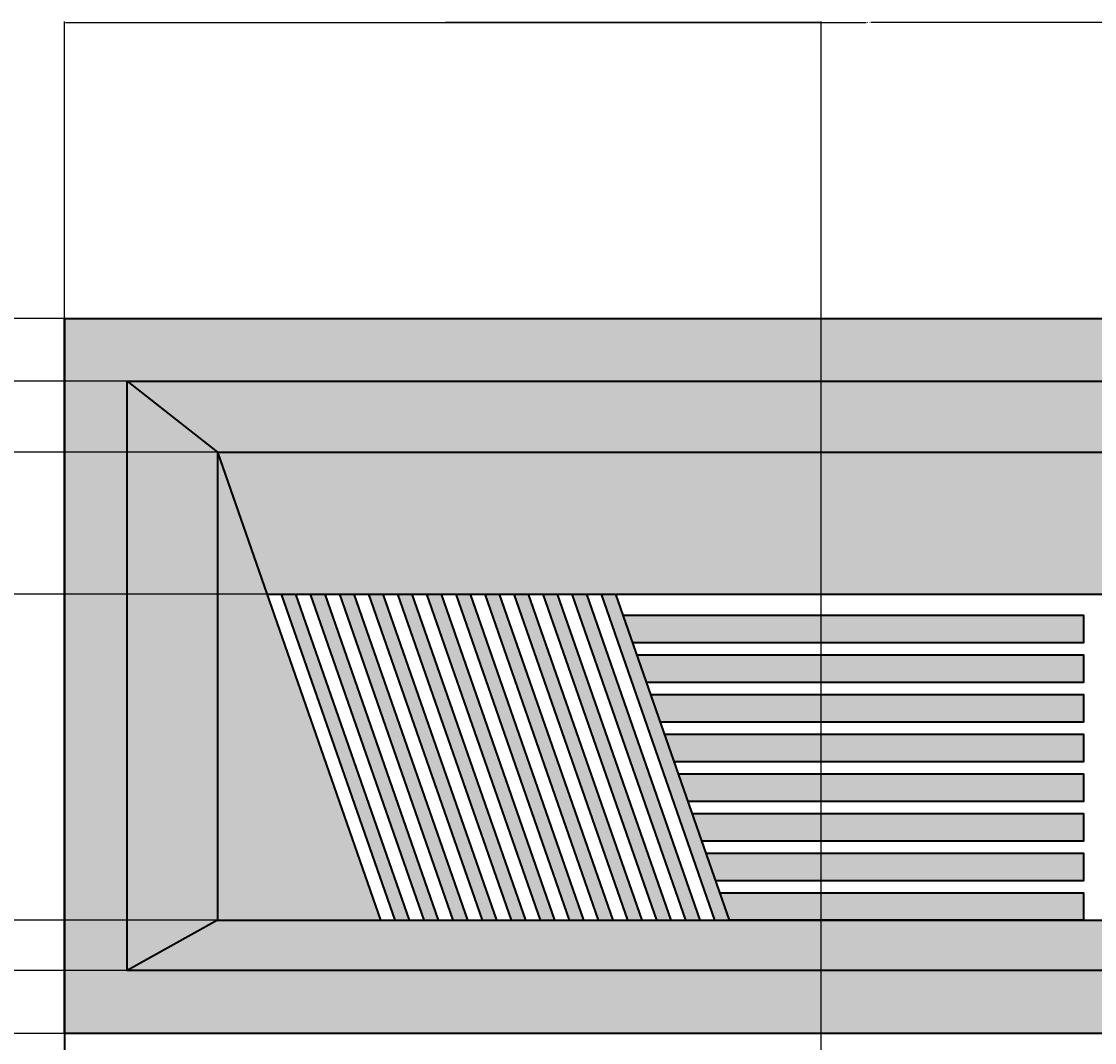
# Model space of a CAD drawing. Units: feet. Extents: x 1141 to 2858, y 751 to 1654.
# Tile 6 of 13: x 1718 to 1916, y 1466 to 1654. Entities that reach past the tile are written whole.
import ezdxf

# ---------------------------------------------------------------- set-up
doc = ezdxf.new("R2010")
doc.units = ezdxf.units.FT
for name, color, linetype, lineweight in [('A-ANNO-DIMS', 2, 'Continuous', 18), ('A-ELEV', 7, 'Continuous', 35), ('A-ELEV-PATT', 8, 'Continuous', 13)]:
    doc.layers.add(name, color=color, linetype=linetype, lineweight=lineweight)
doc.styles.get("Standard").update_dxf_attribs({"font": 'arial.ttf'})
doc.dimstyles.get("Standard").update_dxf_attribs({"dimtxt": 0.18, "dimasz": 0.18, "dimexe": 0.18, "dimexo": 0.0625, "dimgap": 0.09, "dimtad": 0, "dimtih": 1, "dimtoh": 1, "dimdec": 1, "dimzin": 0, "dimdsep": 46, "dimlunit": 3, "dimtxsty": 'Standard', "dimcen": 0.09, "dimadec": 0, "dimazin": 0, "dimtfac": 1, "dimtdec": 1, "dimtofl": 0, "dimtmove": 0, "dimatfit": 3, "dimfxl": 1, "dimtolj": 1, "dimtzin": 0, "dimarcsym": 0})

# ---------------------------------------------------------------- blocks, each defined once
blk = doc.blocks.new('*D24')
at = {"layer": 'A-ANNO-DIMS', "color": 0, "lineweight": -2, "transparency": 16777216}
for p, q in [((1725.97, 1599.45), (1668.14, 1599.45)), ((1668.32, 1599.27), (1668.32, 1202.86)), ((1668.32, 806.08), (1668.32, 1202.49)), ((1725.97, 805.9), (1668.14, 805.9))]:
    blk.add_line(p, q, dxfattribs=at)
at = {"layer": 'A-ANNO-DIMS', "color": 0, "transparency": 16777216}
for points in [[(1668.29, 1599.27), (1668.35, 1599.27), (1668.32, 1599.45)], [(1668.29, 806.08), (1668.35, 806.08), (1668.32, 805.9)]]:
    blk.add_solid(points, dxfattribs=at)
at = {"layer": 'Defpoints', "color": 0, "transparency": 16777216}
for p in [(1668.32, 1599.45), (1726.03, 1599.45), (1726.03, 805.9)]:
    blk.add_point(p, dxfattribs=at)
at = {"layer": 'A-ANNO-DIMS', "color": 0, "transparency": 16777216, "insert": (1668.32, 1202.68), "char_height": 0.18, "attachment_point": 5}
blk.add_mtext('\\A1;793.6', dxfattribs=at)
blk = doc.blocks.new('*D25')
at = {"layer": 'A-ANNO-DIMS', "color": 0, "lineweight": -2, "transparency": 16777216}
for p, q in [((1726.03, 1599.52), (1726.03, 1654.28)), ((1726.21, 1654.1), (1873.98, 1654.1)), ((2022.69, 1654.1), (1874.91, 1654.1)), ((2022.87, 1599.52), (2022.87, 1654.28))]:
    blk.add_line(p, q, dxfattribs=at)
at = {"layer": 'A-ANNO-DIMS', "color": 0, "transparency": 16777216}
for points in [[(1726.21, 1654.13), (1726.21, 1654.07), (1726.03, 1654.1)], [(2022.69, 1654.13), (2022.69, 1654.07), (2022.87, 1654.1)]]:
    blk.add_solid(points, dxfattribs=at)
at = {"layer": 'Defpoints', "color": 0, "transparency": 16777216}
for p in [(2022.87, 1654.1), (1726.03, 1599.45), (2022.87, 1599.45)]:
    blk.add_point(p, dxfattribs=at)
at = {"layer": 'A-ANNO-DIMS', "color": 0, "transparency": 16777216, "insert": (1874.45, 1654.1), "char_height": 0.18, "attachment_point": 5}
blk.add_mtext('\\A1;296.83', dxfattribs=at)
blk = doc.blocks.new('*D39')
at = {"layer": 'A-ANNO-DIMS', "color": 0, "lineweight": -2, "transparency": 16777216}
for p, q in [((2319.24, 1599.45), (1668.14, 1599.45)), ((1668.32, 1599.27), (1668.32, 1202.86)), ((1668.32, 806.08), (1668.32, 1202.49)), ((2319.24, 805.9), (1668.14, 805.9))]:
    blk.add_line(p, q, dxfattribs=at)
at = {"layer": 'A-ANNO-DIMS', "color": 0, "transparency": 16777216}
for points in [[(1668.29, 1599.27), (1668.35, 1599.27), (1668.32, 1599.45)], [(1668.29, 806.08), (1668.35, 806.08), (1668.32, 805.9)]]:
    blk.add_solid(points, dxfattribs=at)
at = {"layer": 'Defpoints', "color": 0, "transparency": 16777216}
for p in [(1668.32, 1599.45), (2319.3, 1599.45), (2319.3, 805.9)]:
    blk.add_point(p, dxfattribs=at)
at = {"layer": 'A-ANNO-DIMS', "color": 0, "transparency": 16777216, "insert": (1668.32, 1202.68), "char_height": 0.18, "attachment_point": 5}
blk.add_mtext('\\A1;793.6', dxfattribs=at)
blk = doc.blocks.new('*D48')
at = {"layer": 'A-ANNO-DIMS', "color": 0, "lineweight": -2, "transparency": 16777216}
for p, q in [((2330.82, 1479.03), (1668.14, 1479.03)), ((1668.32, 1478.85), (1668.32, 1473.42)), ((1668.32, 1467.63), (1668.32, 1473.06)), ((2319.24, 1467.45), (1668.14, 1467.45))]:
    blk.add_line(p, q, dxfattribs=at)
at = {"layer": 'A-ANNO-DIMS', "color": 0, "transparency": 16777216}
for points in [[(1668.29, 1478.85), (1668.35, 1478.85), (1668.32, 1479.03)], [(1668.29, 1467.63), (1668.35, 1467.63), (1668.32, 1467.45)]]:
    blk.add_solid(points, dxfattribs=at)
at = {"layer": 'Defpoints', "color": 0, "transparency": 16777216}
for p in [(1668.32, 1479.03), (2330.88, 1479.03), (2319.3, 1467.45)]:
    blk.add_point(p, dxfattribs=at)
at = {"layer": 'A-ANNO-DIMS', "color": 0, "transparency": 16777216, "insert": (1668.32, 1473.24), "char_height": 0.18, "attachment_point": 5}
blk.add_mtext('\\A1;11.58', dxfattribs=at)
blk = doc.blocks.new('*D49')
at = {"layer": 'A-ANNO-DIMS', "color": 0, "lineweight": -2, "transparency": 16777216}
for p, q in [((2347.45, 1488.33), (1668.14, 1488.33)), ((1668.32, 1488.15), (1668.32, 1483.86)), ((1668.32, 1479.21), (1668.32, 1483.5)), ((2330.82, 1479.03), (1668.14, 1479.03))]:
    blk.add_line(p, q, dxfattribs=at)
at = {"layer": 'A-ANNO-DIMS', "color": 0, "transparency": 16777216}
for points in [[(1668.29, 1488.15), (1668.35, 1488.15), (1668.32, 1488.33)], [(1668.29, 1479.21), (1668.35, 1479.21), (1668.32, 1479.03)]]:
    blk.add_solid(points, dxfattribs=at)
at = {"layer": 'Defpoints', "color": 0, "transparency": 16777216}
for p in [(1668.32, 1488.33), (2347.51, 1488.33), (2330.88, 1479.03)]:
    blk.add_point(p, dxfattribs=at)
at = {"layer": 'A-ANNO-DIMS', "color": 0, "transparency": 16777216, "insert": (1668.32, 1483.68), "char_height": 0.18, "attachment_point": 5}
blk.add_mtext('\\A1;9.293', dxfattribs=at)
blk = doc.blocks.new('*D50')
at = {"layer": 'A-ANNO-DIMS', "color": 0, "lineweight": -2, "transparency": 16777216}
for p, q in [((2356.58, 1548.54), (1668.14, 1548.54)), ((1668.32, 1548.36), (1668.32, 1518.62)), ((1668.32, 1488.51), (1668.32, 1518.25)), ((2347.45, 1488.33), (1668.14, 1488.33))]:
    blk.add_line(p, q, dxfattribs=at)
at = {"layer": 'A-ANNO-DIMS', "color": 0, "transparency": 16777216}
for points in [[(1668.29, 1548.36), (1668.35, 1548.36), (1668.32, 1548.54)], [(1668.29, 1488.51), (1668.35, 1488.51), (1668.32, 1488.33)]]:
    blk.add_solid(points, dxfattribs=at)
at = {"layer": 'Defpoints', "color": 0, "transparency": 16777216}
for p in [(1668.32, 1548.54), (2356.64, 1548.54), (2347.51, 1488.33)]:
    blk.add_point(p, dxfattribs=at)
at = {"layer": 'A-ANNO-DIMS', "color": 0, "transparency": 16777216, "insert": (1668.32, 1518.43), "char_height": 0.18, "attachment_point": 5}
blk.add_mtext('\\A1;60.22', dxfattribs=at)
blk = doc.blocks.new('*D51')
at = {"layer": 'A-ANNO-DIMS', "color": 0, "lineweight": -2, "transparency": 16777216}
for p, q in [((2347.45, 1574.77), (1668.14, 1574.77)), ((1668.32, 1574.59), (1668.32, 1561.84)), ((1668.32, 1548.72), (1668.32, 1561.47)), ((2356.58, 1548.54), (1668.14, 1548.54))]:
    blk.add_line(p, q, dxfattribs=at)
at = {"layer": 'A-ANNO-DIMS', "color": 0, "transparency": 16777216}
for points in [[(1668.29, 1574.59), (1668.35, 1574.59), (1668.32, 1574.77)], [(1668.29, 1548.72), (1668.35, 1548.72), (1668.32, 1548.54)]]:
    blk.add_solid(points, dxfattribs=at)
at = {"layer": 'Defpoints', "color": 0, "transparency": 16777216}
for p in [(1668.32, 1574.77), (2347.51, 1574.77), (2356.64, 1548.54)]:
    blk.add_point(p, dxfattribs=at)
at = {"layer": 'A-ANNO-DIMS', "color": 0, "transparency": 16777216, "insert": (1668.32, 1561.66), "char_height": 0.18, "attachment_point": 5}
blk.add_mtext('\\A1;26.23', dxfattribs=at)
blk = doc.blocks.new('*D52')
at = {"layer": 'A-ANNO-DIMS', "color": 0, "lineweight": -2, "transparency": 16777216}
for p, q in [((2330.82, 1587.87), (1668.14, 1587.87)), ((1668.32, 1587.69), (1668.32, 1581.5)), ((1668.32, 1574.95), (1668.32, 1581.14)), ((2347.45, 1574.77), (1668.14, 1574.77))]:
    blk.add_line(p, q, dxfattribs=at)
at = {"layer": 'A-ANNO-DIMS', "color": 0, "transparency": 16777216}
for points in [[(1668.29, 1587.69), (1668.35, 1587.69), (1668.32, 1587.87)], [(1668.29, 1574.95), (1668.35, 1574.95), (1668.32, 1574.77)]]:
    blk.add_solid(points, dxfattribs=at)
at = {"layer": 'Defpoints', "color": 0, "transparency": 16777216}
for p in [(1668.32, 1587.87), (2330.88, 1587.87), (2347.51, 1574.77)]:
    blk.add_point(p, dxfattribs=at)
at = {"layer": 'A-ANNO-DIMS', "color": 0, "transparency": 16777216, "insert": (1668.32, 1581.32), "char_height": 0.18, "attachment_point": 5}
blk.add_mtext('\\A1;13.102', dxfattribs=at)
blk = doc.blocks.new('*D53')
at = {"layer": 'A-ANNO-DIMS', "color": 0, "lineweight": -2, "transparency": 16777216}
for p, q in [((2319.24, 1599.45), (1668.14, 1599.45)), ((1668.32, 1599.27), (1668.32, 1593.84)), ((1668.32, 1588.05), (1668.32, 1593.48)), ((2330.82, 1587.87), (1668.14, 1587.87))]:
    blk.add_line(p, q, dxfattribs=at)
at = {"layer": 'A-ANNO-DIMS', "color": 0, "transparency": 16777216}
for points in [[(1668.29, 1599.27), (1668.35, 1599.27), (1668.32, 1599.45)], [(1668.29, 1588.05), (1668.35, 1588.05), (1668.32, 1587.87)]]:
    blk.add_solid(points, dxfattribs=at)
at = {"layer": 'Defpoints', "color": 0, "transparency": 16777216}
for p in [(1668.32, 1599.45), (2319.3, 1599.45), (2330.88, 1587.87)]:
    blk.add_point(p, dxfattribs=at)
at = {"layer": 'A-ANNO-DIMS', "color": 0, "transparency": 16777216, "insert": (1668.32, 1593.66), "char_height": 0.18, "attachment_point": 5}
blk.add_mtext('\\A1;11.58', dxfattribs=at)
blk = doc.blocks.new('*D91')
at = {"layer": 'A-ANNO-DIMS', "color": 0, "lineweight": -2, "transparency": 16777216}
for p, q in [((1726.03, 1196.74), (1726.03, 1654.28)), ((1726.21, 1654.1), (1795.4, 1654.1)), ((1865.51, 1654.1), (1796.32, 1654.1)), ((1865.69, 1222.22), (1865.69, 1654.28))]:
    blk.add_line(p, q, dxfattribs=at)
at = {"layer": 'A-ANNO-DIMS', "color": 0, "transparency": 16777216}
for points in [[(1726.21, 1654.13), (1726.21, 1654.07), (1726.03, 1654.1)], [(1865.51, 1654.13), (1865.51, 1654.07), (1865.69, 1654.1)]]:
    blk.add_solid(points, dxfattribs=at)
at = {"layer": 'Defpoints', "color": 0, "transparency": 16777216}
for p in [(1865.69, 1654.1), (1865.69, 1222.16), (1726.03, 1196.68)]:
    blk.add_point(p, dxfattribs=at)
at = {"layer": 'A-ANNO-DIMS', "color": 0, "transparency": 16777216, "insert": (1795.86, 1654.1), "char_height": 0.18, "attachment_point": 5}
blk.add_mtext('\\A1;139.65', dxfattribs=at)

msp = doc.modelspace()

# ---------------------------------------------------------------- hatches: boundary and pattern name
at = {"layer": 'A-ELEV-PATT'}
h = msp.add_hatch(color=256, dxfattribs=at)
h.dxf.hatch_style = 1
h.paths.add_polyline_path([(2206.032, 1599.4527), (2192.689, 1599.4527), (2192.689, 919.339), (2206.032, 919.339)])
h.paths.add_polyline_path([(2190.2416, 1599.4527), (2175.463, 1599.4527), (2175.463, 919.339), (2190.2416, 919.339)])
h.paths.add_polyline_path([(2173.0156, 1599.4527), (2117.407, 1599.4527), (2117.407, 919.339), (2173.0156, 919.339)])
h.paths.add_polyline_path([(2022.8666, 1057.9008), (1726.032, 1057.9008), (1726.032, 925.9008), (2022.8666, 925.9008)])
h.paths.add_polyline_path([(1737.6123, 937.4811), (1737.6123, 1046.3205), (2011.2863, 1046.3205), (2011.2863, 937.4811)], flags=16)
h.paths.add_polyline_path([(1754.2423, 946.7736), (1754.2423, 1033.2183), (2004.2323, 1033.2183), (2004.2323, 946.7736), (2004.3069, 946.6754), (1906.0824, 946.6754)], flags=0)
h.paths.add_polyline_path([(1900.5421, 946.7736), (1857.5566, 946.7736), (1857.5566, 1033.2183), (1900.5421, 1033.2183)], flags=0)
h.paths.add_polyline_path([(1910.8368, 951.4297), (1910.8368, 1022.7957), (1999.478, 1022.7957), (1999.478, 951.4297)], flags=0)
h.paths.add_polyline_path([(1930.8039, 951.4297), (1930.8039, 1022.7957), (1932.373, 1022.7957), (1932.373, 951.4297)], flags=0)
h.paths.add_polyline_path([(1851.6414, 946.7736), (1826.5664, 946.7736), (1826.5664, 967.8234), (1793.4402, 967.8234), (1793.4402, 946.7736), (1790.4043, 946.7736), (1790.4043, 967.8234), (1754.2423, 967.8234), (1754.2423, 970.4796), (1790.4043, 970.4796), (1790.4043, 1033.2183), (1793.4402, 1033.2183), (1793.4402, 970.4796), (1826.5664, 970.4796), (1826.5664, 1033.2183), (1851.6414, 1033.2183)], flags=0)
h.paths.add_polyline_path([(1954.3728, 951.4297), (1954.3728, 1022.7957), (1955.9419, 1022.7957), (1955.9419, 951.4297)], flags=0)
h.paths.add_polyline_path([(1977.7327, 951.4297), (1977.7327, 1022.7957), (1979.3018, 1022.7957), (1979.3018, 951.4297)], flags=0)
h.paths.add_polyline_path([(2022.8666, 1193.2888), (1726.032, 1193.2888), (1726.032, 1061.2888), (2022.8666, 1061.2888)])
h.paths.add_polyline_path([(1737.6123, 1072.869), (1737.6123, 1181.7085), (2011.2863, 1181.7085), (2011.2863, 1072.869)], flags=16)
h.paths.add_polyline_path([(1754.2423, 1082.1616), (1754.2423, 1168.6063), (2004.2323, 1168.6063), (2004.2323, 1082.1616), (2004.3069, 1082.0634), (1906.0824, 1082.0634)], flags=0)
h.paths.add_polyline_path([(1900.5421, 1082.1616), (1857.5566, 1082.1616), (1857.5566, 1168.6063), (1900.5421, 1168.6063)], flags=0)
h.paths.add_polyline_path([(1910.8368, 1086.8177), (1910.8368, 1158.1837), (1999.478, 1158.1837), (1999.478, 1086.8177)], flags=0)
h.paths.add_polyline_path([(1930.8039, 1086.8177), (1930.8039, 1158.1837), (1932.373, 1158.1837), (1932.373, 1086.8177)], flags=0)
h.paths.add_polyline_path([(1851.6414, 1082.1616), (1826.5664, 1082.1616), (1826.5664, 1103.2114), (1793.4402, 1103.2114), (1793.4402, 1082.1616), (1790.4043, 1082.1616), (1790.4043, 1103.2114), (1754.2423, 1103.2114), (1754.2423, 1105.8676), (1790.4043, 1105.8676), (1790.4043, 1168.6063), (1793.4402, 1168.6063), (1793.4402, 1105.8676), (1826.5664, 1105.8676), (1826.5664, 1168.6063), (1851.6414, 1168.6063)], flags=0)
h.paths.add_polyline_path([(1954.3728, 1086.8177), (1954.3728, 1158.1837), (1955.9419, 1158.1837), (1955.9419, 1086.8177)], flags=0)
h.paths.add_polyline_path([(1977.7327, 1086.8177), (1977.7327, 1158.1837), (1979.3018, 1158.1837), (1979.3018, 1086.8177)], flags=0)
h.paths.add_polyline_path([(2022.8666, 1599.4527), (1726.032, 1599.4527), (1726.032, 1467.4527), (2022.8666, 1467.4527)])
h.paths.add_polyline_path([(2011.2863, 1479.033), (1737.6123, 1479.033), (1737.6123, 1587.8725), (2011.2863, 1587.8725)], flags=16)
h.paths.add_polyline_path([(2004.2323, 1488.3255), (1754.2423, 1488.3255), (1754.2423, 1574.7702), (2004.2323, 1574.7702)], flags=0)
h.paths.add_polyline_path([(1829.1345, 1544.6458), (1914.1177, 1544.6458), (1914.1177, 1539.5463), (1830.9097, 1539.5463), (1831.6817, 1537.3286), (1914.1177, 1537.3286), (1914.1177, 1532.2291), (1833.4569, 1532.2291), (1834.229, 1530.0113), (1914.1177, 1530.0113), (1914.1177, 1524.9118), (1836.0042, 1524.9118), (1836.7762, 1522.694), (1914.1177, 1522.694), (1914.1177, 1517.5946), (1838.5514, 1517.5946), (1839.3235, 1515.3768), (1914.1177, 1515.3768), (1914.1177, 1510.2773), (1841.0987, 1510.2773), (1841.8707, 1508.0595), (1914.1177, 1508.0595), (1914.1177, 1502.9601), (1843.6459, 1502.9601), (1844.4179, 1500.7423), (1914.1177, 1500.7423), (1914.1177, 1495.6428), (1846.1931, 1495.6428), (1846.9652, 1493.425), (1914.1177, 1493.425), (1914.1177, 1488.3255), (1848.6593, 1488.3255), (1848.6593, 1488.5583)], flags=0)
h.paths.add_polyline_path([(2117.407, 1464.0647), (1820.5724, 1464.0647), (1820.5724, 1332.0647), (2117.407, 1332.0647)])
h.paths.add_polyline_path([(2105.8267, 1452.4845), (2105.8267, 1343.645), (1832.1527, 1343.645), (1832.1527, 1452.4845)], flags=16)
h.paths.add_polyline_path([(2089.1967, 1439.3822), (2089.1967, 1352.9376), (1937.3566, 1352.9376), (1937.3566, 1352.8393), (1839.1321, 1352.8393), (1839.2067, 1352.9376), (1839.2067, 1439.3822), (1937.3566, 1439.3822)], flags=0)
h.paths.add_polyline_path([(2016.8727, 1439.3822), (2016.8727, 1376.6436), (2049.9988, 1376.6436), (2049.9988, 1439.3822), (2053.0347, 1439.3822), (2053.0347, 1376.6436), (2089.1967, 1376.6436), (2089.1967, 1373.9873), (2053.0347, 1373.9873), (2053.0347, 1352.9376), (2049.9988, 1352.9376), (2049.9988, 1373.9873), (2016.8727, 1373.9873), (2016.8727, 1352.9376), (1991.7976, 1352.9376), (1991.7976, 1439.3822)], flags=0)
h.paths.add_polyline_path([(1985.8824, 1439.3822), (1985.8824, 1352.9376), (1942.8969, 1352.9376), (1942.8969, 1439.3822)], flags=0)
h.paths.add_polyline_path([(1932.6022, 1428.9596), (1932.6022, 1357.5937), (1843.961, 1357.5937), (1843.961, 1428.9596)], flags=0)
h.paths.add_polyline_path([(1912.6351, 1428.9596), (1912.6351, 1357.5937), (1911.066, 1357.5937), (1911.066, 1428.9596)], flags=0)
h.paths.add_polyline_path([(1889.0662, 1428.9596), (1889.0662, 1357.5937), (1887.4971, 1357.5937), (1887.4971, 1428.9596)], flags=0)
h.paths.add_polyline_path([(1865.7063, 1428.9596), (1865.7063, 1357.5937), (1864.1372, 1357.5937), (1864.1372, 1428.9596)], flags=0)
h.paths.add_polyline_path([(2117.407, 1328.6768), (1820.5724, 1328.6768), (1820.5724, 1196.6768), (2117.407, 1196.6768)])
h.paths.add_polyline_path([(2105.8267, 1317.0965), (2105.8267, 1208.257), (1832.1527, 1208.257), (1832.1527, 1317.0965)], flags=16)
h.paths.add_polyline_path([(2089.1967, 1303.9943), (2089.1967, 1217.5496), (1937.3566, 1217.5496), (1937.3566, 1217.4513), (1839.1321, 1217.4513), (1839.2067, 1217.5496), (1839.2067, 1303.9943), (1937.3566, 1303.9943)], flags=0)
h.paths.add_polyline_path([(2016.8727, 1303.9943), (2016.8727, 1241.2556), (2049.9988, 1241.2556), (2049.9988, 1303.9943), (2053.0347, 1303.9943), (2053.0347, 1241.2556), (2089.1967, 1241.2556), (2089.1967, 1238.5993), (2053.0347, 1238.5993), (2053.0347, 1217.5496), (2049.9988, 1217.5496), (2049.9988, 1238.5993), (2016.8727, 1238.5993), (2016.8727, 1217.5496), (1991.7976, 1217.5496), (1991.7976, 1303.9943)], flags=0)
h.paths.add_polyline_path([(1985.8824, 1303.9943), (1985.8824, 1217.5496), (1942.8969, 1217.5496), (1942.8969, 1303.9943)], flags=0)
h.paths.add_polyline_path([(1932.6022, 1293.5716), (1932.6022, 1222.2057), (1843.961, 1222.2057), (1843.961, 1293.5716)], flags=0)
h.paths.add_polyline_path([(1912.6351, 1293.5716), (1912.6351, 1222.2057), (1911.066, 1222.2057), (1911.066, 1293.5716)], flags=0)
h.paths.add_polyline_path([(1889.0662, 1293.5716), (1889.0662, 1222.2057), (1887.4971, 1222.2057), (1887.4971, 1293.5716)], flags=0)
h.paths.add_polyline_path([(1865.7063, 1293.5716), (1865.7063, 1222.2057), (1864.1372, 1222.2057), (1864.1372, 1293.5716)], flags=0)
h.paths.add_polyline_path([(2206.032, 917.3598), (2027.2589, 917.3598), (2027.2589, 805.9008), (2206.032, 805.9008)])
h.paths.add_polyline_path([(1852.1771, 917.3598), (1726.032, 917.3598), (1726.032, 805.9008), (1852.1771, 805.9008)])
h.paths.add_polyline_path([(2063.3101, 1580.3829), (2093.938, 1580.3829), (2093.938, 1513.0494), (2063.3101, 1513.0494)])
h.paths.add_polyline_path([(2063.3101, 1580.3829), (2093.938, 1580.3829), (2093.938, 1513.0494), (2063.3101, 1513.0494)])
h = msp.add_hatch(color=256, dxfattribs=at)
h.dxf.hatch_style = 1
h.paths.add_polyline_path([(2011.2863, 1587.8725), (1737.6123, 1587.8725), (1754.2423, 1574.7702), (2004.2323, 1574.7702)])
h.paths.add_polyline_path([(1754.2423, 1574.7702), (1737.6123, 1587.8725), (1737.6123, 1479.033), (1754.2423, 1488.3255)])
h.paths.add_polyline_path([(2011.2863, 1587.8725), (2004.2323, 1574.7702), (2004.2323, 1488.3255), (2011.2863, 1479.033)])
h.paths.add_polyline_path([(2004.2323, 1488.3255), (1754.2423, 1488.3255), (1737.6123, 1479.033), (2011.2863, 1479.033)])
h.paths.add_polyline_path([(2105.8267, 1452.4845), (1832.1527, 1452.4845), (1839.2067, 1439.3822), (1937.3566, 1439.3822), (2089.1967, 1439.3822)])
h.paths.add_polyline_path([(1839.2067, 1439.3822), (1832.1527, 1452.4845), (1832.1527, 1343.645), (1839.2067, 1352.9376)])
h.paths.add_polyline_path([(2105.8267, 1452.4845), (2089.1967, 1439.3822), (2089.1967, 1352.9376), (2105.8267, 1343.645)])
h.paths.add_polyline_path([(2089.1967, 1352.9376), (1937.3566, 1352.9376), (1937.3566, 1352.8393), (1839.1321, 1352.8393), (1832.1527, 1343.645), (2105.8267, 1343.645)])
h.paths.add_polyline_path([(1942.8969, 1439.3822), (1937.3566, 1439.3822), (1937.3566, 1352.9376), (1942.8969, 1352.9376)])
h.paths.add_polyline_path([(1991.7976, 1439.3822), (1985.8824, 1439.3822), (1985.8824, 1352.9376), (1991.7976, 1352.9376)])
h.paths.add_polyline_path([(2109.4211, 1591.4669), (2030.8524, 1591.4669), (2030.8524, 1580.3829), (2093.938, 1580.3829)])
h.paths.add_polyline_path([(2109.4211, 1591.4669), (2093.938, 1580.3829), (2093.938, 1475.4386), (2109.4211, 1475.4386)])
h.paths.add_polyline_path([(1991.7976, 1303.9943), (1985.8824, 1303.9943), (1985.8824, 1217.5496), (1991.7976, 1217.5496)])
h.paths.add_polyline_path([(1942.8969, 1303.9943), (1937.3566, 1303.9943), (1937.3566, 1217.5496), (1942.8969, 1217.5496)])
h.paths.add_polyline_path([(2105.8267, 1317.0965), (1832.1527, 1317.0965), (1839.2067, 1303.9943), (1937.3566, 1303.9943), (2089.1967, 1303.9943)])
h.paths.add_polyline_path([(1839.2067, 1303.9943), (1832.1527, 1317.0965), (1832.1527, 1208.257), (1839.2067, 1217.5496)])
h.paths.add_polyline_path([(2089.1967, 1217.5496), (1937.3566, 1217.5496), (1937.3566, 1217.4513), (1839.1321, 1217.4513), (1832.1527, 1208.257), (2105.8267, 1208.257)])
h.paths.add_polyline_path([(2105.8267, 1317.0965), (2089.1967, 1303.9943), (2089.1967, 1217.5496), (2105.8267, 1208.257)])
h.paths.add_polyline_path([(1754.2423, 1168.6063), (1737.6123, 1181.7085), (1737.6123, 1072.869), (1754.2423, 1082.1616)])
h.paths.add_polyline_path([(2011.2863, 1181.7085), (1737.6123, 1181.7085), (1754.2423, 1168.6063), (2004.2323, 1168.6063)])
h.paths.add_polyline_path([(2011.2863, 1181.7085), (2004.2323, 1168.6063), (2004.2323, 1082.1616), (2011.2863, 1072.869)])
h.paths.add_polyline_path([(2004.3069, 1082.0634), (1906.0824, 1082.0634), (1754.2423, 1082.1616), (1737.6123, 1072.869), (2011.2863, 1072.869)])
h.paths.add_polyline_path([(1906.0824, 1168.6063), (1900.5421, 1168.6063), (1900.5421, 1082.1616), (1906.0824, 1082.1616)])
h.paths.add_polyline_path([(1857.5566, 1168.6063), (1851.6414, 1168.6063), (1851.6414, 1082.1616), (1857.5566, 1082.1616)])
h.paths.add_polyline_path([(1906.0824, 1033.2183), (1900.5421, 1033.2183), (1900.5421, 946.7736), (1906.0824, 946.7736)])
h.paths.add_polyline_path([(1857.5566, 1033.2183), (1851.6414, 1033.2183), (1851.6414, 946.7736), (1857.5566, 946.7736)])
h.paths.add_polyline_path([(1754.2423, 1033.2183), (1737.6123, 1046.3205), (1737.6123, 937.4811), (1754.2423, 946.7736)])
h.paths.add_polyline_path([(2011.2863, 1046.3205), (1737.6123, 1046.3205), (1754.2423, 1033.2183), (2004.2323, 1033.2183)])
h.paths.add_polyline_path([(2011.2863, 1046.3205), (2004.2323, 1033.2183), (2004.2323, 946.7736), (2011.2863, 937.4811)])
h.paths.add_polyline_path([(2004.3069, 946.6754), (1906.0824, 946.6754), (1754.2423, 946.7736), (1737.6123, 937.4811), (2011.2863, 937.4811)])
h.paths.add_polyline_path([(2175.463, 1599.4527), (2173.0156, 1599.4527), (2173.0156, 919.339), (2175.463, 919.339)])
h = msp.add_hatch(color=256, dxfattribs=at)
h.dxf.hatch_style = 1
h.paths.add_polyline_path([(2004.2323, 1574.7702), (1754.2423, 1574.7702), (1763.3732, 1548.5407), (1979.2491, 1548.5407), (1979.2491, 1488.3255), (2004.2323, 1488.3255)])
h.paths.add_polyline_path([(1754.2423, 1574.7702), (1754.2423, 1488.3255), (1784.3349, 1488.3255)], flags=17)
h.paths.add_polyline_path([(1768.7403, 1548.5407), (1766.0183, 1548.5407), (1786.98, 1488.3255), (1789.702, 1488.3255)], flags=17)
h.paths.add_polyline_path([(1774.1074, 1548.5407), (1771.3854, 1548.5407), (1792.3471, 1488.3255), (1795.0692, 1488.3255)], flags=17)
h.paths.add_polyline_path([(1779.4746, 1548.5407), (1776.7525, 1548.5407), (1797.7142, 1488.3255), (1800.4363, 1488.3255)], flags=17)
h.paths.add_polyline_path([(1784.8417, 1548.5407), (1782.1197, 1548.5407), (1803.0814, 1488.3255), (1805.8034, 1488.3255)], flags=17)
h.paths.add_polyline_path([(1790.2088, 1548.5407), (1787.4868, 1548.5407), (1808.4485, 1488.3255), (1811.1705, 1488.3255)], flags=17)
h.paths.add_polyline_path([(1795.5759, 1548.5407), (1792.8539, 1548.5407), (1813.8156, 1488.3255), (1816.5376, 1488.3255)], flags=17)
h.paths.add_polyline_path([(1800.9431, 1548.5407), (1798.221, 1548.5407), (1819.1827, 1488.3255), (1821.9048, 1488.3255)], flags=17)
h.paths.add_polyline_path([(1806.3102, 1548.5407), (1803.5881, 1548.5407), (1824.5499, 1488.3255), (1827.2719, 1488.3255)], flags=17)
h.paths.add_polyline_path([(1811.6773, 1548.5407), (1808.9553, 1548.5407), (1829.917, 1488.3255), (1832.639, 1488.3255)], flags=17)
h.paths.add_polyline_path([(1817.0444, 1548.5407), (1814.3224, 1548.5407), (1835.2841, 1488.3255), (1838.0061, 1488.3255)], flags=17)
h.paths.add_polyline_path([(1822.4115, 1548.5407), (1819.6895, 1548.5407), (1840.6512, 1488.3255), (1843.3733, 1488.3255)], flags=17)
h.paths.add_polyline_path([(1827.7787, 1548.5407), (1825.0566, 1548.5407), (1846.0183, 1488.3255), (1848.6593, 1488.3255), (1848.6593, 1488.5583)], flags=17)
h.paths.add_polyline_path([(1914.1177, 1544.6458), (1829.1345, 1544.6458), (1830.9097, 1539.5463), (1914.1177, 1539.5463)], flags=17)
h.paths.add_polyline_path([(1914.1177, 1537.3286), (1831.6817, 1537.3286), (1833.4569, 1532.2291), (1914.1177, 1532.2291)], flags=17)
h.paths.add_polyline_path([(1914.1177, 1530.0113), (1834.229, 1530.0113), (1836.0042, 1524.9118), (1914.1177, 1524.9118)], flags=17)
h.paths.add_polyline_path([(1914.1177, 1522.694), (1836.7762, 1522.694), (1838.5514, 1517.5946), (1914.1177, 1517.5946)], flags=17)
h.paths.add_polyline_path([(1914.1177, 1515.3768), (1839.3235, 1515.3768), (1841.0987, 1510.2773), (1914.1177, 1510.2773)], flags=17)
h.paths.add_polyline_path([(1914.1177, 1508.0595), (1841.8707, 1508.0595), (1843.6459, 1502.9601), (1914.1177, 1502.9601)], flags=17)
h.paths.add_polyline_path([(1914.1177, 1500.7423), (1844.4179, 1500.7423), (1846.1931, 1495.6428), (1914.1177, 1495.6428)], flags=17)
h.paths.add_polyline_path([(1914.1177, 1493.425), (1846.9652, 1493.425), (1848.7404, 1488.3255), (1914.1177, 1488.3255)], flags=17)
h.paths.add_polyline_path([(1920.7331, 1548.5407), (1918.1624, 1548.5407), (1918.3509, 1488.3255), (1920.9216, 1488.3255)], flags=17)
h.paths.add_polyline_path([(1925.8019, 1548.5407), (1923.2312, 1548.5407), (1923.4197, 1488.3255), (1925.9904, 1488.3255)], flags=17)
h.paths.add_polyline_path([(1930.8708, 1548.5407), (1928.3, 1548.5407), (1928.4885, 1488.3255), (1931.0592, 1488.3255)], flags=17)
h.paths.add_polyline_path([(1935.9396, 1548.5407), (1933.3688, 1548.5407), (1933.5573, 1488.3255), (1936.128, 1488.3255)], flags=17)
h.paths.add_polyline_path([(1941.0084, 1548.5407), (1938.4376, 1548.5407), (1938.6261, 1488.3255), (1941.1968, 1488.3255)], flags=17)
h.paths.add_polyline_path([(1946.0772, 1548.5407), (1943.5064, 1548.5407), (1943.6949, 1488.3255), (1946.2656, 1488.3255)], flags=17)
h.paths.add_polyline_path([(1951.146, 1548.5407), (1948.5752, 1548.5407), (1948.7637, 1488.3255), (1951.3344, 1488.3255)], flags=17)
h.paths.add_polyline_path([(1956.2148, 1548.5407), (1953.644, 1548.5407), (1953.8325, 1488.3255), (1956.4032, 1488.3255)], flags=17)
h.paths.add_polyline_path([(1961.2836, 1548.5407), (1958.7128, 1548.5407), (1958.9013, 1488.3255), (1961.472, 1488.3255)], flags=17)
h.paths.add_polyline_path([(1966.3524, 1548.5407), (1963.7816, 1548.5407), (1963.9701, 1488.3255), (1966.5408, 1488.3255)], flags=17)
h.paths.add_polyline_path([(1971.4212, 1548.5407), (1968.8504, 1548.5407), (1969.0389, 1488.3255), (1971.6096, 1488.3255)], flags=17)
h.paths.add_polyline_path([(1976.49, 1548.5407), (1973.9192, 1548.5407), (1974.1077, 1488.3255), (1976.6784, 1488.3255)], flags=17)
h.paths.add_polyline_path([(2027.2589, 914.5568), (1852.1771, 914.5568), (1852.1771, 909.9657), (2027.2589, 909.9657)])
h.paths.add_polyline_path([(2027.2589, 906.8659), (1852.1771, 906.8659), (1852.1771, 902.2747), (2027.2589, 902.2747)])
h.paths.add_polyline_path([(2027.2589, 899.1749), (1852.1771, 899.1749), (1852.1771, 894.5837), (2027.2589, 894.5837)])
h.paths.add_polyline_path([(2027.2589, 891.4839), (1852.1771, 891.4839), (1852.1771, 886.8927), (2027.2589, 886.8927)])
h.paths.add_polyline_path([(2027.2589, 883.793), (1852.1771, 883.793), (1852.1771, 879.2018), (2027.2589, 879.2018)])
h.paths.add_polyline_path([(2027.2589, 876.102), (1852.1771, 876.102), (1852.1771, 871.5108), (2027.2589, 871.5108)])
h.paths.add_polyline_path([(2027.2589, 868.411), (1852.1771, 868.411), (1852.1771, 863.8198), (2027.2589, 863.8198)])
h.paths.add_polyline_path([(2027.2589, 860.72), (1852.1771, 860.72), (1852.1771, 856.1289), (2027.2589, 856.1289)])
h.paths.add_polyline_path([(2027.2589, 853.0291), (1852.1771, 853.0291), (1852.1771, 848.4379), (2027.2589, 848.4379)])
h.paths.add_polyline_path([(2027.2589, 845.3381), (1852.1771, 845.3381), (1852.1771, 840.7469), (2027.2589, 840.7469)])
h.paths.add_polyline_path([(2027.2589, 837.6471), (1852.1771, 837.6471), (1852.1771, 833.056), (2027.2589, 833.056)])
h.paths.add_polyline_path([(2027.2589, 829.9562), (1852.1771, 829.9562), (1852.1771, 825.365), (2027.2589, 825.365)])
h.paths.add_polyline_path([(2027.2589, 822.2652), (1852.1771, 822.2652), (1852.1771, 817.674), (2027.2589, 817.674)])
h.paths.add_polyline_path([(2027.2589, 814.5742), (1852.1771, 814.5742), (1852.1771, 809.983), (2027.2589, 809.983)])

# ---------------------------------------------------------------- linework, layer by layer
at = {"layer": 'A-ELEV'}
for p, q in [((1726.032, 1599.4527), (1726.032, 919.339)), ((1726.032, 1599.4527), (1726.032, 919.339)), ((1737.6123, 1587.8725), (1754.2423, 1574.7702)), ((1737.6123, 1587.8725), (1754.2423, 1574.7702)), ((1754.2423, 1574.7702), (1754.2423, 1488.3255)), ((1754.2423, 1574.7702), (2004.2323, 1574.7702)), ((1754.2423, 1574.7702), (1784.3349, 1488.3255)), ((1754.2423, 1574.7702), (1754.2423, 1488.3255)), ((1754.2423, 1574.7702), (2004.2323, 1574.7702)), ((1754.2423, 1574.7702), (1784.3349, 1488.3255)), ((1763.3732, 1548.5407), (1979.2491, 1548.5407)), ((1763.3732, 1548.5407), (1979.2491, 1548.5407)), ((1754.2423, 1488.3255), (1737.6123, 1479.033)), ((1754.2423, 1488.3255), (1737.6123, 1479.033)), ((1754.2423, 1488.3255), (2004.2323, 1488.3255)), ((1754.2423, 1488.3255), (2004.2323, 1488.3255))]:
    msp.add_line(p, q, dxfattribs=at)
for points in [[(1726.032, 1599.4527), (2022.8666, 1599.4527), (2022.8666, 1467.4527), (1726.032, 1467.4527)], [(1726.032, 1599.4527), (2022.8666, 1599.4527), (2022.8666, 1467.4527), (1726.032, 1467.4527)], [(1737.6123, 1587.8725), (2011.2863, 1587.8725), (2011.2863, 1479.033), (1737.6123, 1479.033)], [(1737.6123, 1587.8725), (2011.2863, 1587.8725), (2011.2863, 1479.033), (1737.6123, 1479.033)]]:
    msp.add_lwpolyline(points, close=True, dxfattribs=at)
for points in [[(1766.0183, 1548.5407), (1786.98, 1488.3255)], [(1766.0183, 1548.5407), (1786.98, 1488.3255)], [(1789.702, 1488.3255), (1768.7403, 1548.5407)], [(1789.702, 1488.3255), (1768.7403, 1548.5407)], [(1771.3854, 1548.5407), (1792.3471, 1488.3255)], [(1771.3854, 1548.5407), (1792.3471, 1488.3255)], [(1795.0692, 1488.3255), (1774.1074, 1548.5407)], [(1795.0692, 1488.3255), (1774.1074, 1548.5407)], [(1776.7525, 1548.5407), (1797.7142, 1488.3255)], [(1776.7525, 1548.5407), (1797.7142, 1488.3255)], [(1800.4363, 1488.3255), (1779.4746, 1548.5407)], [(1800.4363, 1488.3255), (1779.4746, 1548.5407)], [(1782.1197, 1548.5407), (1803.0814, 1488.3255)], [(1782.1197, 1548.5407), (1803.0814, 1488.3255)], [(1805.8034, 1488.3255), (1784.8417, 1548.5407)], [(1805.8034, 1488.3255), (1784.8417, 1548.5407)], [(1787.4868, 1548.5407), (1808.4485, 1488.3255)], [(1787.4868, 1548.5407), (1808.4485, 1488.3255)], [(1811.1705, 1488.3255), (1790.2088, 1548.5407)], [(1811.1705, 1488.3255), (1790.2088, 1548.5407)], [(1792.8539, 1548.5407), (1813.8156, 1488.3255)], [(1792.8539, 1548.5407), (1813.8156, 1488.3255)], [(1816.5376, 1488.3255), (1795.5759, 1548.5407)], [(1816.5376, 1488.3255), (1795.5759, 1548.5407)], [(1798.221, 1548.5407), (1819.1827, 1488.3255)], [(1798.221, 1548.5407), (1819.1827, 1488.3255)], [(1821.9048, 1488.3255), (1800.9431, 1548.5407)], [(1821.9048, 1488.3255), (1800.9431, 1548.5407)], [(1803.5881, 1548.5407), (1824.5499, 1488.3255)], [(1803.5881, 1548.5407), (1824.5499, 1488.3255)], [(1827.2719, 1488.3255), (1806.3102, 1548.5407)], [(1827.2719, 1488.3255), (1806.3102, 1548.5407)], [(1808.9553, 1548.5407), (1829.917, 1488.3255)], [(1808.9553, 1548.5407), (1829.917, 1488.3255)], [(1832.639, 1488.3255), (1811.6773, 1548.5407)], [(1832.639, 1488.3255), (1811.6773, 1548.5407)], [(1814.3224, 1548.5407), (1835.2841, 1488.3255)], [(1814.3224, 1548.5407), (1835.2841, 1488.3255)], [(1838.0061, 1488.3255), (1817.0444, 1548.5407)], [(1838.0061, 1488.3255), (1817.0444, 1548.5407)], [(1819.6895, 1548.5407), (1840.6512, 1488.3255)], [(1819.6895, 1548.5407), (1840.6512, 1488.3255)], [(1843.3733, 1488.3255), (1822.4115, 1548.5407)], [(1843.3733, 1488.3255), (1822.4115, 1548.5407)], [(1825.0566, 1548.5407), (1846.0183, 1488.3255)], [(1825.0566, 1548.5407), (1846.0183, 1488.3255)], [(1848.7404, 1488.3255), (1827.7787, 1548.5407)], [(1848.7404, 1488.3255), (1827.7787, 1548.5407)], [(1829.1345, 1544.6458), (1914.1177, 1544.6458), (1914.1177, 1539.5463), (1830.9097, 1539.5463)], [(1829.1345, 1544.6458), (1914.1177, 1544.6458), (1914.1177, 1539.5463), (1830.9097, 1539.5463)], [(1831.6817, 1537.3286), (1914.1177, 1537.3286), (1914.1177, 1532.2291), (1833.4569, 1532.2291)], [(1831.6817, 1537.3286), (1914.1177, 1537.3286), (1914.1177, 1532.2291), (1833.4569, 1532.2291)], [(1834.229, 1530.0113), (1914.1177, 1530.0113), (1914.1177, 1524.9118), (1836.0042, 1524.9118)], [(1834.229, 1530.0113), (1914.1177, 1530.0113), (1914.1177, 1524.9118), (1836.0042, 1524.9118)], [(1836.7762, 1522.694), (1914.1177, 1522.694), (1914.1177, 1517.5946), (1838.5514, 1517.5946)], [(1836.7762, 1522.694), (1914.1177, 1522.694), (1914.1177, 1517.5946), (1838.5514, 1517.5946)], [(1839.3235, 1515.3768), (1914.1177, 1515.3768), (1914.1177, 1510.2773), (1841.0987, 1510.2773)], [(1839.3235, 1515.3768), (1914.1177, 1515.3768), (1914.1177, 1510.2773), (1841.0987, 1510.2773)], [(1841.8707, 1508.0595), (1914.1177, 1508.0595), (1914.1177, 1502.9601), (1843.6459, 1502.9601)], [(1841.8707, 1508.0595), (1914.1177, 1508.0595), (1914.1177, 1502.9601), (1843.6459, 1502.9601)], [(1844.4179, 1500.7423), (1914.1177, 1500.7423), (1914.1177, 1495.6428), (1846.1931, 1495.6428)], [(1844.4179, 1500.7423), (1914.1177, 1500.7423), (1914.1177, 1495.6428), (1846.1931, 1495.6428)], [(1846.9652, 1493.425), (1914.1177, 1493.425), (1914.1177, 1488.3255), (1848.6593, 1488.3255), (1848.6593, 1488.5583)], [(1846.9652, 1493.425), (1914.1177, 1493.425), (1914.1177, 1488.3255), (1848.6593, 1488.3255), (1848.6593, 1488.5583)]]:
    msp.add_lwpolyline(points, dxfattribs=at)

# ---------------------------------------------------------------- dimensions: what is measured, and where the dimension line sits
at = {"layer": 'A-ANNO-DIMS'}
for base, p1, p2, picture, middle in [((2022.8666, 1654.1027), (1726.032, 1599.4527), (2022.8666, 1599.4527), '*D25', (1874.4493, 1654.1027)), ((1865.6863, 1654.1027), (1726.032, 1196.6768), (1865.6863, 1222.1557), '*D91', (1795.8592, 1654.1027))]:
    dim = msp.add_linear_dim(base=base, p1=p1, p2=p2, dimstyle='Standard', override={"dimdec": 2, "dimlfac": 1, "dimrnd": 0, "dimzin": 0, "dimdsep": 46, "dimlunit": 2}, dxfattribs=at)
    dim.commit()
    dim.dimension.update_dxf_attribs({"geometry": picture, "text_midpoint": middle})
for base, p1, p2, override, picture, middle in [((1668.3207, 1599.4527), (1726.032, 805.9008), (1726.032, 1599.4527), {"dimdec": 1, "dimlfac": 1, "dimrnd": 0, "dimzin": 0, "dimdsep": 46, "dimlunit": 2}, '*D24', (1668.3207, 1202.6768)), ((1668.3207, 1599.4527), (2319.3013, 805.9008), (2319.3013, 1599.4527), {"dimdec": 1, "dimlfac": 1, "dimrnd": 0, "dimzin": 0, "dimdsep": 46, "dimlunit": 2}, '*D39', (1668.3207, 1202.6768)), ((1668.3207, 1599.4527), (2330.8815, 1587.8725), (2319.3013, 1599.4527), {"dimdec": 2, "dimlfac": 1, "dimrnd": 0, "dimzin": 0, "dimdsep": 46, "dimlunit": 2}, '*D53', (1668.3207, 1593.6626)), ((1668.3207, 1587.8725), (2347.5116, 1574.7702), (2330.8815, 1587.8725), {"dimdec": 3, "dimlfac": 1, "dimrnd": 0, "dimzin": 0, "dimdsep": 46, "dimlunit": 2}, '*D52', (1668.3207, 1581.3214)), ((1668.3207, 1574.7702), (2356.6424, 1548.5407), (2347.5116, 1574.7702), {"dimdec": 2, "dimlfac": 1, "dimrnd": 0, "dimzin": 0, "dimdsep": 46, "dimlunit": 2}, '*D51', (1668.3207, 1561.6555)), ((1668.3207, 1548.5407), (2347.5116, 1488.3255), (2356.6424, 1548.5407), {"dimdec": 2, "dimlfac": 1, "dimrnd": 0, "dimzin": 0, "dimdsep": 46, "dimlunit": 2}, '*D50', (1668.3207, 1518.4331)), ((1668.32065, 1488.32554), (2330.88152, 1479.03299), (2347.51155, 1488.32554), {"dimdec": 3, "dimlfac": 1, "dimrnd": 0, "dimzin": 0, "dimdsep": 46, "dimlunit": 2}, '*D49', (1668.32065, 1483.67926)), ((1668.3207, 1479.033), (2319.3013, 1467.4527), (2330.8815, 1479.033), {"dimdec": 2, "dimlfac": 1, "dimrnd": 0, "dimzin": 0, "dimdsep": 46, "dimlunit": 2}, '*D48', (1668.3207, 1473.2429))]:
    dim = msp.add_linear_dim(base=base, p1=p1, p2=p2, angle=90, dimstyle='Standard', override=override, dxfattribs=at)
    dim.commit()
    dim.dimension.update_dxf_attribs({"geometry": picture, "text_midpoint": middle})

doc.saveas('drawing.dxf')
